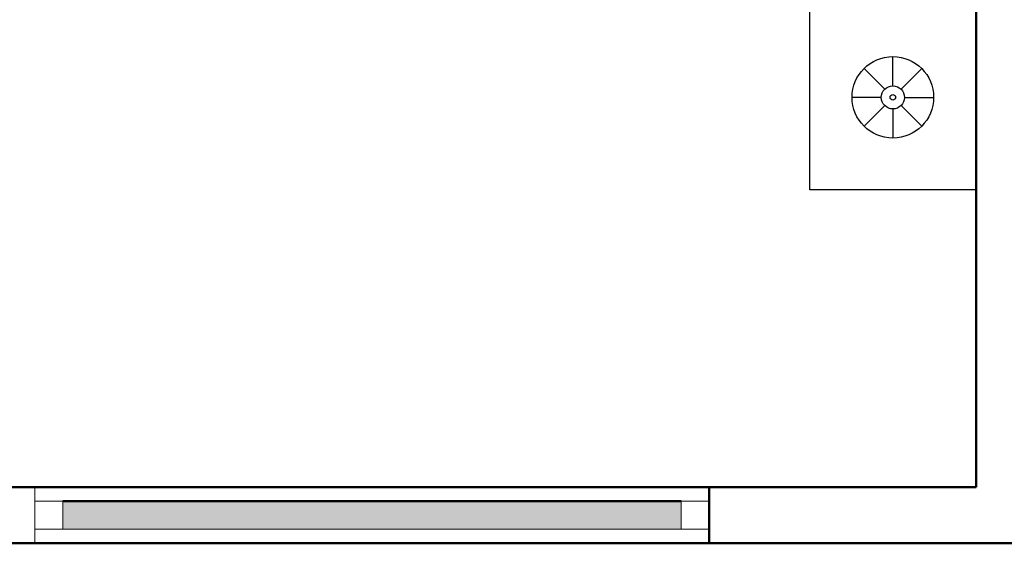
# Model space of a CAD drawing. Units: inches. Extents: x 3064 to 19385, y 846 to 15425.
# Tile 12 of 108: x 3680 to 3785, y 976 to 1032. Entities that reach past the tile are written whole.
import ezdxf

# ---------------------------------------------------------------- set-up
doc = ezdxf.new("R2010")
doc.units = ezdxf.units.IN
for name, color, linetype, lineweight in [('A-FLOR-FIXT', 9, 'Continuous', 18), ('A-GLAZ', 4, 'Continuous', 18), ('A-WALL', 7, 'Continuous', 50)]:
    doc.layers.add(name, color=color, linetype=linetype, lineweight=lineweight)
doc.layers.add('BLOCK', color=6, linetype='Continuous')

# ---------------------------------------------------------------- blocks, each defined once
blk = doc.blocks.new('A$C52E67D0D')
at = {"layer": 'BLOCK'}
for p, q in [((2251.5, 1605.5), (2251.5, 1684.7)), ((2229.3, 1596.3), (2173.3, 1652.3)), ((2273.7, 1596.3), (2329.7, 1652.3)), ((2220.1, 1574.1), (2140.9, 1574.1)), ((2229.3, 1551.9), (2173.3, 1495.9)), ((2273.7, 1551.9), (2329.7, 1495.9)), ((2282.9, 1574.1), (2362.1, 1574.1)), ((2251.5, 1542.8), (2251.5, 1463.5))]:
    blk.add_line(p, q, dxfattribs=at)
blk.add_lwpolyline([(2001, 1348.6), (2001, 1799.6), (2502, 1799.6), (2502, 1348.6)], close=True, dxfattribs=at)
for radius in [110.6, 31.4, 7.46]:
    blk.add_circle((2251.5, 1574.1), radius, dxfattribs=at)
blk = doc.blocks.new('WIN-1900')
blk.add_line((3, 0), (3, 66))
blk.add_lwpolyline([(3, 66), (0, 66), (0, 69), (3, 69)], close=True)

msp = doc.modelspace()

# ---------------------------------------------------------------- hatches: boundary and pattern name
at = {"layer": 'A-GLAZ'}
h = msp.add_hatch(color=256, dxfattribs=at)
h.dxf.hatch_style = 1
h.paths.add_polyline_path([(3684.86, 980.84), (3684.86, 977.84), (3750.86, 977.84), (3750.86, 980.84)])

# ---------------------------------------------------------------- linework, layer by layer
msp.add_line((3681.86, 976.34), (3681.86, 982.34), dxfattribs=at)
msp.add_lwpolyline([(3681.86, 977.84), (3681.86, 980.84), (3684.86, 980.84), (3684.86, 977.84)], close=True, dxfattribs=at)
at = {"layer": 'A-WALL'}
for p, q in [((3782.36, 1144.34), (3782.36, 982.34)), ((3782.36, 982.34), (3653.36, 982.34)), ((3753.86, 976.34), (3753.86, 982.34)), ((3684.86, 980.84), (3750.86, 980.84)), ((3989.36, 976.34), (3647.36, 976.34))]:
    msp.add_line(p, q, dxfattribs=at)

# ---------------------------------------------------------------- block references
at = {"layer": 'A-FLOR-FIXT', "xscale": 0.039370099999992, "yscale": 0.039370099999992, "zscale": 0.039370099999992, "rotation": 270}
msp.add_blockref('A$C52E67D0D', (3711.49, 1112.59), dxfattribs=at)
at = {"layer": 'A-GLAZ', "rotation": 269.9999999999995}
msp.add_blockref('WIN-1900', (3684.86, 980.84), dxfattribs=at)

doc.saveas('drawing.dxf')
